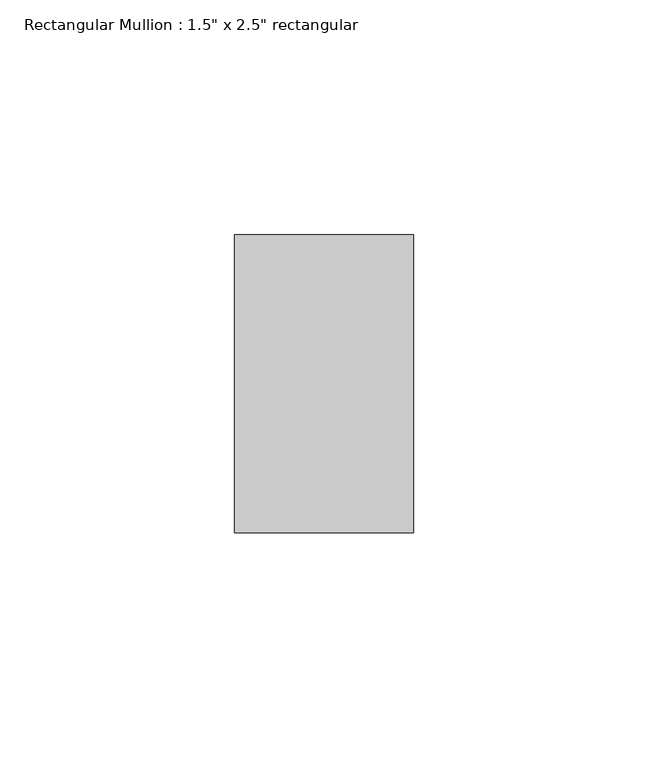
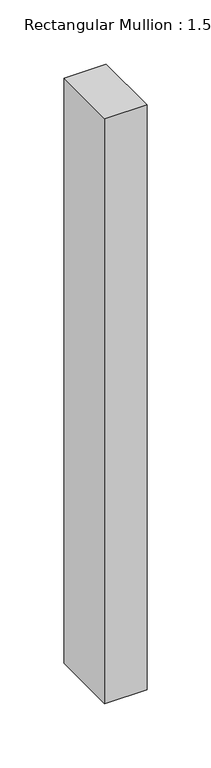
"""IFC4 building model written with IfcOpenShell, lengths in millimetres: member geometry."""

from ifc_helpers import new_model, si_unit, frame, origin, place, context, project, spatial, polyline, outline, extrude, source, transform, mapped, element, save


def member_494741c6(model_context):
    return source(origin(), model_context, "Body", "SweptSolid", [
        extrude(outline(polyline([(19.05, 31.75), (19.05, -31.75), (-19.05, -31.75), (-19.05, 31.75), (19.05, 31.75)])), frame((0.0, 0.0, -557.1903046), z_axis=(0.0, 0.0, 1.0), x_axis=(1.0, 0.0, 0.0)), (0.0, 0.0, 1.0), 557.1903046),
    ])


if __name__ == "__main__":
    model = new_model("IFC4")
    model_context = context("Model", 3, world=origin())
    ifc_project = project(units=[si_unit("LENGTHUNIT", "METRE", prefix="MILLI")], contexts=[model_context])
    site = spatial("IfcSite", under=ifc_project)
    building = spatial("IfcBuilding", under=site)
    placement = place(None, origin())
    member_shape = member_494741c6(model_context)
    element("IfcMember", 1, ObjectType="Rectangular Mullion : 1.5\" x 2.5\" rectangular", at=placement, inside=building, context=model_context, shape_type="MappedRepresentation", body=[
        mapped(member_shape, transform((0.0, 0.0, 0.0), x_axis=(1.0, 0.0, 0.0), y_axis=(0.0, 1.0, 0.0), z_axis=(0.0, 0.0, 1.0))),
    ])
    save(model, "model.ifc")

# Revit data of these elements
# Type "Rectangular Mullion : 1.5\" x 2.5\" rectangular"
#   built-in parameter 1007304 = 0.208333 (stored number, unit not read)
#   built-in parameter 1007301 = 0.0625 (stored number, unit not read)
#   built-in parameter 1007300 = 0.0625 (stored number, unit not read)
# Element 1 (IfcMember, "Rectangular Mullion : 1.5\" x 2.5\" rectangular")
#   Materials on its faces: "Leather - Black"
# Materials
#   "Leather - Black": class "Generic", colour RGB 40 40 40, transparency 0, Cost = 0
